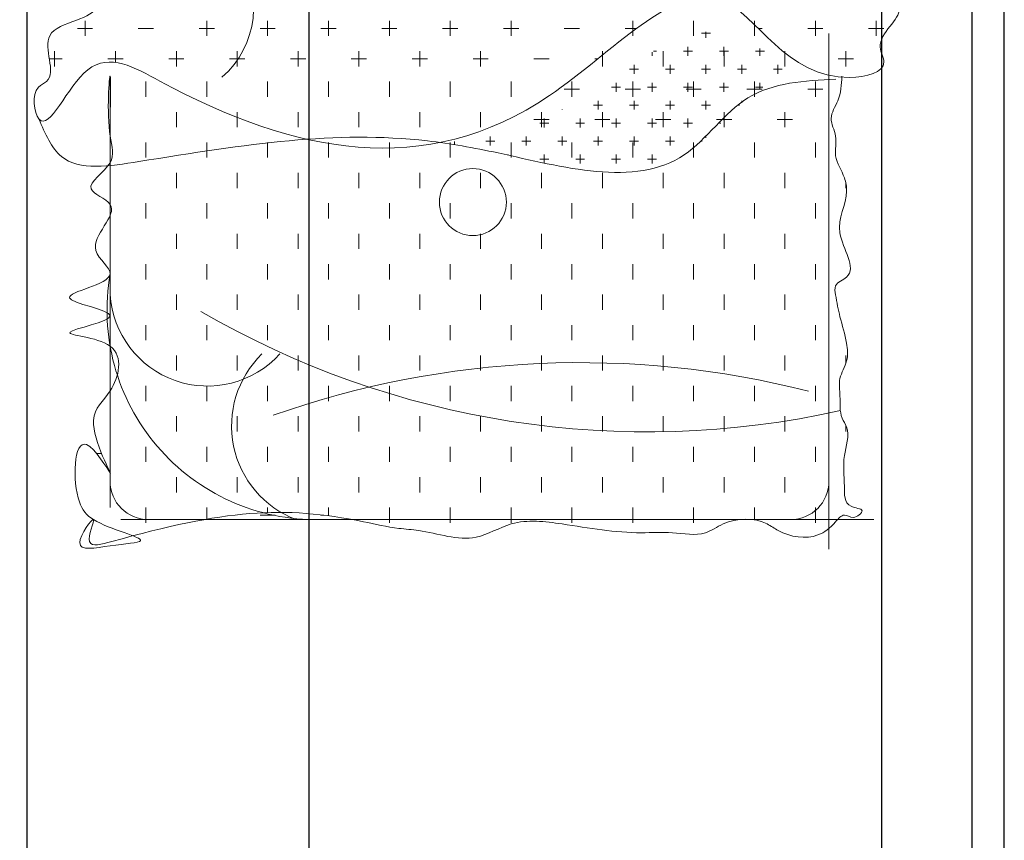
# Model space of a CAD drawing. Units: inches. Extents: x -438 to 102, y -60 to 1091.
# Tile 16 of 20: x -68 to 13, y 699 to 766. Entities that reach past the tile are written whole.
import ezdxf

# ---------------------------------------------------------------- set-up
doc = ezdxf.new("R2010")
doc.units = ezdxf.units.IN
doc.header["$MEASUREMENT"] = 0
doc.layers.add('A-ANNO-DIMS', color=217, linetype='Continuous', lineweight=18, true_color=0x93278f)
doc.layers.add('Furniture', color=7, linetype='Continuous', lineweight=15)
doc.styles.get("Standard").update_dxf_attribs({"font": 'arial.ttf'})
doc.dimstyles.get("Standard").update_dxf_attribs({"dimtxt": 8, "dimasz": 0.18, "dimexe": 0.18, "dimexo": 0.0625, "dimgap": 0.09, "dimtad": 0, "dimtih": 1, "dimtoh": 1, "dimdec": 4, "dimzin": 0, "dimdsep": 46, "dimlunit": 3, "dimtxsty": 'Standard', "dimcen": 0.09, "dimadec": 0, "dimazin": 0, "dimtfac": 1, "dimtdec": 4, "dimtofl": 0, "dimtmove": 0, "dimatfit": 3, "dimfxl": 1, "dimtolj": 1, "dimtzin": 0, "dimarcsym": 0})

# ---------------------------------------------------------------- blocks, each defined once
blk = doc.blocks.new('BED-DOUBLE-WITH-NIGHTSTANDS')
for p, q in [((-31.218, -41.19), (-31.218, -39.94)), ((-21.218, -41.19), (-21.218, -39.94)), ((-16.218, -41.19), (-16.218, -39.94)), ((-11.218, -41.19), (-11.218, -39.94)), ((-6.218, -41.19), (-6.218, -39.94)), ((-1.218, -41.19), (-1.218, -39.94)), ((3.782, -41.19), (3.782, -39.94)), ((13.782, -41.19), (13.782, -39.94)), ((18.782, -41.19), (18.782, -39.94)), ((23.782, -41.19), (23.782, -39.94)), ((28.782, -41.19), (28.782, -39.94)), ((33.782, -41.19), (33.782, -39.94)), ((-30.593, -40.565), (-31.843, -40.565)), ((-25.593, -40.565), (-26.843, -40.565)), ((-20.593, -40.565), (-21.843, -40.565)), ((-15.593, -40.565), (-16.843, -40.565)), ((-10.593, -40.565), (-11.843, -40.565)), ((-5.593, -40.565), (-6.843, -40.565)), ((-0.593, -40.565), (-1.843, -40.565)), ((4.407, -40.565), (3.157, -40.565)), ((9.407, -40.565), (8.157, -40.565)), ((14.104, -40.565), (13.157, -40.565)), ((20.164, -40.972), (19.426, -40.972)), ((19.795, -41.341), (19.795, -40.863)), ((24.407, -40.565), (24.086, -40.565)), ((29.407, -40.565), (28.157, -40.565)), ((29.898, -40.998), (29.898, -83.358)), ((34.407, -40.565), (33.157, -40.565)), ((-33.718, -43.69), (-33.718, -42.44)), ((-28.718, -43.367), (-28.718, -42.44)), ((-23.718, -43.69), (-23.718, -42.44)), ((-18.718, -43.69), (-18.718, -42.44)), ((-13.718, -43.69), (-13.718, -42.44)), ((-8.718, -43.69), (-8.718, -42.44)), ((-3.718, -43.69), (-3.718, -42.44)), ((1.282, -43.69), (1.282, -42.44)), ((11.282, -43.69), (11.282, -42.44)), ((15.366, -42.817), (15.366, -42.522)), ((15.735, -42.448), (15.495, -42.448)), ((16.282, -43.69), (16.282, -42.44)), ((18.688, -42.448), (17.949, -42.448)), ((18.318, -42.817), (18.318, -42.079)), ((21.64, -42.448), (20.902, -42.448)), ((21.271, -42.817), (21.271, -42.079)), ((21.282, -43.69), (21.282, -42.44)), ((24.593, -42.448), (23.855, -42.448)), ((24.224, -42.817), (24.224, -42.225)), ((26.282, -43.69), (26.282, -42.44)), ((31.282, -43.69), (31.282, -42.44)), ((-33.093, -43.065), (-34.154, -43.065)), ((-28.093, -43.065), (-29.343, -43.065)), ((-23.093, -43.065), (-24.343, -43.065)), ((-18.093, -43.065), (-19.343, -43.065)), ((-13.093, -43.065), (-14.343, -43.065)), ((-8.093, -43.065), (-9.343, -43.065)), ((-3.093, -43.065), (-4.343, -43.065)), ((1.907, -43.065), (0.657, -43.065)), ((6.907, -43.065), (5.657, -43.065)), ((10.916, -43.065), (10.657, -43.065)), ((13.889, -44.294), (13.889, -43.555)), ((16.842, -44.294), (16.842, -43.555)), ((19.795, -44.294), (19.795, -43.555)), ((22.748, -44.294), (22.748, -43.555)), ((25.7, -44.294), (25.7, -43.555)), ((31.907, -43.065), (30.657, -43.065)), ((14.258, -43.924), (13.52, -43.924)), ((17.211, -43.924), (16.473, -43.924)), ((20.164, -43.924), (19.426, -43.924)), ((23.117, -43.924), (22.378, -43.924)), ((26.069, -43.924), (25.331, -43.924)), ((-29.157, -79.94), (-29.157, -44.493)), ((-26.218, -46.19), (-26.218, -44.94)), ((-21.218, -46.19), (-21.218, -44.94)), ((-16.218, -46.19), (-16.218, -44.94)), ((-11.218, -46.19), (-11.218, -44.94)), ((-6.218, -46.19), (-6.218, -44.94)), ((-1.218, -46.19), (-1.218, -44.94)), ((3.782, -46.19), (3.782, -44.94)), ((8.782, -46.19), (8.782, -44.94)), ((12.413, -45.77), (12.413, -45.032)), ((13.782, -46.19), (13.782, -44.94)), ((15.366, -45.77), (15.366, -45.032)), ((18.318, -45.77), (18.318, -45.032)), ((18.782, -46.19), (18.782, -44.94)), ((21.271, -45.77), (21.271, -45.032)), ((23.782, -46.19), (23.782, -44.94)), ((24.224, -45.56), (24.224, -45.032)), ((28.782, -46.19), (28.782, -44.94)), ((9.407, -45.565), (8.157, -45.565)), ((12.782, -45.401), (12.044, -45.401)), ((14.407, -45.565), (13.157, -45.565)), ((15.735, -45.401), (14.997, -45.401)), ((18.688, -45.401), (17.949, -45.401)), ((19.407, -45.565), (18.157, -45.565)), ((21.64, -45.401), (20.902, -45.401)), ((24.407, -45.565), (23.157, -45.565)), ((24.466, -45.401), (23.855, -45.401)), ((29.407, -45.565), (28.157, -45.565)), ((11.306, -46.877), (10.567, -46.877)), ((10.937, -47.246), (10.937, -46.508)), ((14.258, -46.877), (13.52, -46.877)), ((13.889, -47.246), (13.889, -46.508)), ((17.211, -46.877), (16.473, -46.877)), ((16.842, -47.246), (16.842, -46.508)), ((20.164, -46.877), (19.426, -46.877)), ((19.795, -47.246), (19.795, -46.508)), ((22.546, -46.877), (22.378, -46.877)), ((22.748, -46.697), (22.748, -46.508)), ((-23.718, -48.69), (-23.718, -47.44)), ((-18.718, -48.69), (-18.718, -47.44)), ((-13.718, -48.69), (-13.718, -47.44)), ((-8.718, -48.69), (-8.718, -47.44)), ((-3.718, -48.69), (-3.718, -47.44)), ((1.282, -48.69), (1.282, -47.44)), ((6.282, -48.69), (6.282, -47.44)), ((7.984, -47.246), (7.984, -47.199)), ((11.282, -48.69), (11.282, -47.44)), ((16.282, -48.69), (16.282, -47.44)), ((21.282, -48.69), (21.282, -47.44)), ((26.282, -48.69), (26.282, -47.44)), ((-34.327, -48.065), (-34.343, -48.065)), ((6.907, -48.065), (5.657, -48.065)), ((6.877, -48.354), (6.138, -48.354)), ((6.507, -48.723), (6.507, -47.984)), ((9.829, -48.354), (9.091, -48.354)), ((9.46, -48.723), (9.46, -47.984)), ((11.907, -48.065), (10.657, -48.065)), ((12.782, -48.354), (12.044, -48.354)), ((12.413, -48.723), (12.413, -47.984)), ((15.735, -48.354), (14.997, -48.354)), ((15.366, -48.723), (15.366, -47.984)), ((16.907, -48.065), (15.657, -48.065)), ((18.688, -48.354), (17.949, -48.354)), ((18.318, -48.723), (18.318, -47.984)), ((21.907, -48.065), (20.657, -48.065)), ((21.024, -48.354), (20.902, -48.354)), ((21.271, -48.106), (21.271, -47.984)), ((26.907, -48.065), (25.657, -48.065)), ((-26.218, -51.19), (-26.218, -49.94)), ((-21.218, -51.19), (-21.218, -49.94)), ((-16.218, -51.19), (-16.218, -49.94)), ((-11.218, -51.19), (-11.218, -49.94)), ((-6.218, -51.19), (-6.218, -49.94)), ((-1.218, -51.19), (-1.218, -49.94)), ((-0.874, -50.112), (-0.874, -49.874)), ((2.447, -49.83), (1.709, -49.83)), ((2.078, -50.199), (2.078, -49.461)), ((3.782, -51.19), (3.782, -49.94)), ((5.4, -49.83), (4.662, -49.83)), ((5.031, -50.199), (5.031, -49.461)), ((8.353, -49.83), (7.615, -49.83)), ((7.984, -50.199), (7.984, -49.461)), ((8.782, -51.19), (8.782, -49.94)), ((11.306, -49.83), (10.567, -49.83)), ((10.937, -50.199), (10.937, -49.461)), ((14.258, -49.83), (13.52, -49.83)), ((13.782, -51.19), (13.782, -49.94)), ((13.889, -50.199), (13.889, -49.461)), ((17.211, -49.83), (16.473, -49.83)), ((16.842, -50.199), (16.842, -49.461)), ((18.782, -51.19), (18.782, -49.94)), ((19.485, -49.83), (19.426, -49.83)), ((19.795, -49.55), (19.795, -49.461)), ((23.782, -51.19), (23.782, -49.94)), ((28.782, -51.19), (28.782, -49.94)), ((3.555, -50.987), (3.555, -50.937)), ((6.507, -51.614), (6.507, -50.937)), ((9.46, -51.675), (9.46, -50.937)), ((12.413, -51.675), (12.413, -50.937)), ((15.366, -51.675), (15.366, -50.937)), ((6.877, -51.306), (6.138, -51.306)), ((9.829, -51.306), (9.091, -51.306)), ((12.782, -51.306), (12.044, -51.306)), ((15.735, -51.306), (14.997, -51.306)), ((-23.718, -53.69), (-23.718, -52.44)), ((-18.718, -53.69), (-18.718, -52.44)), ((-13.718, -53.69), (-13.718, -52.44)), ((-8.718, -53.69), (-8.718, -52.44)), ((-3.718, -53.69), (-3.718, -52.44)), ((1.282, -53.69), (1.282, -52.44)), ((6.282, -53.69), (6.282, -52.44)), ((11.282, -53.69), (11.282, -52.44)), ((16.282, -53.69), (16.282, -52.44)), ((21.282, -53.69), (21.282, -52.44)), ((26.282, -53.69), (26.282, -52.44)), ((31.282, -53.69), (31.282, -53.251)), ((-26.218, -56.19), (-26.218, -54.94)), ((-21.218, -56.19), (-21.218, -54.94)), ((-16.218, -56.19), (-16.218, -54.94)), ((-11.218, -56.19), (-11.218, -54.94)), ((-6.218, -56.19), (-6.218, -54.94)), ((-1.218, -56.19), (-1.218, -54.94)), ((3.782, -56.19), (3.782, -54.94)), ((8.782, -56.19), (8.782, -54.94)), ((13.782, -56.19), (13.782, -54.94)), ((18.782, -56.19), (18.782, -54.94)), ((23.782, -56.19), (23.782, -54.94)), ((28.782, -56.19), (28.782, -54.94)), ((-23.718, -58.69), (-23.718, -57.44)), ((-18.718, -58.69), (-18.718, -57.44)), ((-13.718, -58.69), (-13.718, -57.44)), ((-8.718, -58.69), (-8.718, -57.44)), ((-3.718, -58.69), (-3.718, -57.44)), ((1.282, -58.69), (1.282, -57.44)), ((6.282, -58.69), (6.282, -57.44)), ((11.282, -58.69), (11.282, -57.44)), ((16.282, -58.69), (16.282, -57.44)), ((21.282, -58.69), (21.282, -57.44)), ((26.282, -58.69), (26.282, -57.44)), ((-26.218, -61.19), (-26.218, -59.94)), ((-21.218, -61.19), (-21.218, -59.94)), ((-16.218, -61.19), (-16.218, -59.94)), ((-11.218, -61.19), (-11.218, -59.94)), ((-6.218, -61.19), (-6.218, -59.94)), ((-1.218, -61.19), (-1.218, -59.94)), ((3.782, -61.19), (3.782, -59.94)), ((8.782, -61.19), (8.782, -59.94)), ((13.782, -61.19), (13.782, -59.94)), ((18.782, -61.19), (18.782, -59.94)), ((23.782, -61.19), (23.782, -59.94)), ((28.782, -61.19), (28.782, -59.94)), ((-23.718, -63.69), (-23.718, -62.44)), ((-18.718, -63.69), (-18.718, -62.44)), ((-13.718, -63.69), (-13.718, -62.44)), ((-8.718, -63.69), (-8.718, -62.44)), ((-3.718, -63.69), (-3.718, -62.44)), ((1.282, -63.69), (1.282, -62.44)), ((6.282, -63.69), (6.282, -62.44)), ((11.282, -63.69), (11.282, -62.44)), ((16.282, -63.69), (16.282, -62.44)), ((21.282, -63.69), (21.282, -62.44)), ((26.282, -63.69), (26.282, -62.44)), ((-26.218, -66.19), (-26.218, -64.94)), ((-21.218, -66.19), (-21.218, -64.94)), ((-16.218, -66.19), (-16.218, -64.94)), ((-11.218, -66.19), (-11.218, -64.94)), ((-6.218, -66.19), (-6.218, -64.94)), ((-1.218, -66.19), (-1.218, -64.94)), ((3.782, -66.19), (3.782, -64.94)), ((8.782, -66.19), (8.782, -64.94)), ((13.782, -66.19), (13.782, -64.94)), ((18.782, -66.19), (18.782, -64.94)), ((23.782, -66.19), (23.782, -64.94)), ((28.782, -66.19), (28.782, -64.94)), ((-23.718, -68.69), (-23.718, -67.44)), ((-18.718, -68.69), (-18.718, -67.44)), ((-13.718, -68.69), (-13.718, -67.44)), ((-8.718, -68.69), (-8.718, -67.44)), ((-3.718, -68.69), (-3.718, -67.44)), ((1.282, -68.69), (1.282, -67.44)), ((6.282, -68.69), (6.282, -67.44)), ((11.282, -68.69), (11.282, -67.44)), ((16.282, -68.69), (16.282, -67.44)), ((21.282, -68.69), (21.282, -67.44)), ((26.282, -68.69), (26.282, -67.44)), ((31.282, -68.103), (31.282, -67.44)), ((-26.218, -71.19), (-26.218, -69.94)), ((-21.218, -71.19), (-21.218, -69.94)), ((-16.218, -71.19), (-16.218, -69.94)), ((-11.218, -71.19), (-11.218, -69.94)), ((-6.218, -71.19), (-6.218, -69.94)), ((-1.218, -71.19), (-1.218, -69.94)), ((3.782, -71.19), (3.782, -69.94)), ((8.782, -71.19), (8.782, -69.94)), ((13.782, -71.19), (13.782, -69.94)), ((18.782, -71.19), (18.782, -69.94)), ((23.782, -71.19), (23.782, -69.94)), ((28.782, -71.19), (28.782, -69.94)), ((-23.718, -73.69), (-23.718, -72.44)), ((-18.718, -73.69), (-18.718, -72.44)), ((-13.718, -73.69), (-13.718, -72.44)), ((-8.718, -73.69), (-8.718, -72.44)), ((-3.718, -73.69), (-3.718, -72.44)), ((1.282, -73.69), (1.282, -72.44)), ((6.282, -73.69), (6.282, -72.44)), ((11.282, -73.69), (11.282, -72.44)), ((16.282, -73.69), (16.282, -72.44)), ((21.282, -73.69), (21.282, -72.44)), ((26.282, -73.69), (26.282, -72.44)), ((31.282, -73.69), (31.282, -73.162)), ((-26.218, -76.19), (-26.218, -74.94)), ((-21.218, -76.19), (-21.218, -74.94)), ((-16.218, -76.19), (-16.218, -74.94)), ((-11.218, -76.19), (-11.218, -74.94)), ((-6.218, -76.19), (-6.218, -74.94)), ((-1.218, -76.19), (-1.218, -74.94)), ((3.782, -76.19), (3.782, -74.94)), ((8.782, -76.19), (8.782, -74.94)), ((13.782, -76.19), (13.782, -74.94)), ((18.782, -76.19), (18.782, -74.94)), ((23.782, -76.19), (23.782, -74.94)), ((28.782, -76.19), (28.782, -74.94)), ((-29.87, -75.491), (-30.279, -75.491)), ((-23.718, -78.69), (-23.718, -77.44)), ((-18.718, -78.69), (-18.718, -77.44)), ((-13.718, -78.69), (-13.718, -77.44)), ((-8.718, -78.69), (-8.718, -77.44)), ((-3.718, -78.69), (-3.718, -77.44)), ((1.282, -78.69), (1.282, -77.44)), ((6.282, -78.69), (6.282, -77.44)), ((11.282, -78.69), (11.282, -77.44)), ((16.282, -78.69), (16.282, -77.44)), ((21.282, -78.69), (21.282, -77.44)), ((26.282, -78.69), (26.282, -77.44)), ((-26.218, -81.19), (-26.218, -79.94)), ((-21.218, -80.893), (-21.218, -79.94)), ((-16.218, -80.354), (-16.218, -79.94)), ((-11.218, -80.612), (-11.218, -79.94)), ((-6.218, -81.19), (-6.218, -79.94)), ((-1.218, -81.19), (-1.218, -79.94)), ((3.782, -81.19), (3.782, -79.94)), ((8.782, -81.19), (8.782, -79.94)), ((13.782, -81.19), (13.782, -79.94)), ((18.782, -81.19), (18.782, -79.94)), ((23.782, -80.944), (23.782, -79.94)), ((28.782, -81.19), (28.782, -79.94)), ((-15.593, -80.565), (-16.843, -80.565)), ((-11.59, -80.565), (-11.843, -80.565)), ((33.596, -80.928), (-28.288, -80.928))]:
    blk.add_line(p, q)
blk.add_circle((0.643, -54.842), 2.753)
for centre, radius, start, end in [((-24.929, -38.89), 7.557, 311.04012, 36.13845), ((-12.201, -63.717), 17.214, 170.06779, 270.93205), ((-21.159, -61.944), 8.013, 183.53609, 317.84857), ((14.986, -0.753), 72.965, 239.8126, 282.54723), ((-10.938, -73.228), 8.244, 134.23532, 249.05847), ((9.498, -143.884), 75.853, 75.71433, 109.44594), ((-26.01, -77.778), 3.15, 180, 270), ((26.749, -77.778), 3.15, 270, 0)]:
    blk.add_arc(centre, radius, start, end)
for points, knots in [([(31.925, -25.289), (32.572, -26.623), (33.591, -28.721), (30.294, -29.708), (31.006, -32.636), (33.349, -32.829), (32.919, -35.123), (30.078, -36.111), (33.789, -37.483), (36.776, -39.184), (33.388, -41.323), (35.068, -44.058), (26.871, -46.019), (20.992, -32.347), (2.098, -54.118), (-16.077, -50.434), (-31.165, -41.37), (-34.819, -50.791), (-35.745, -45.559), (-33.272, -44.571), (-36.072, -39.916), (-29.615, -39.911), (-31.051, -37.176), (-31.793, -35.409), (-31.667, -30.426), (-16.859, -30.756), (-35.732, -24.414), (-25.676, -23.879), (-16.82, -24.973), (2.336, -26.688), (17.46, -24.9), (30.087, -22.482), (31.544, -24.706), (31.925, -25.289)], [0, 0, 0, 0, 3.481099, 5.475811, 8.043407, 9.436812, 11.330727, 12.888379, 16.258255, 18.252967, 21.734596, 23.018392, 26.087149, 38.445812, 54.5649, 86.600283, 92.594507, 98.286547, 100.905288, 101.70342, 105.471876, 109.954916, 110.954151, 113.598333, 116.114301, 124.231953, 133.25029, 137.509046, 143.991555, 164.906349, 189.961005, 195.579007, 197.573325, 197.573325, 197.573325, 197.573325]), ([(30.963, -44.508), (30.926, -45.187), (30.862, -46.385), (29.771, -47.932), (30.68, -49.438), (30.181, -51.195), (31.183, -52.546), (31.556, -54.753), (29.857, -57.224), (32.609, -60.735), (30.283, -61.502), (30.515, -62.875), (30.787, -64.379), (31.375, -66.149), (31.511, -67.951), (30.622, -69.27), (30.889, -70.902), (30.721, -72.32), (31.738, -73.744), (30.928, -75.806), (31.246, -77.781), (31.095, -79.972), (33.091, -80.014), (31.893, -81.001), (31.103, -80.322), (30.205, -81.428), (28.73, -82.665), (26.29, -82.307), (24.174, -80.727), (21.697, -80.779), (19.495, -82.403), (17.064, -81.884), (13.167, -82.166), (8.822, -81.359), (4.068, -80.767), (0.461, -83.087), (-2.79, -81.846), (-5.869, -81.655), (-14.296, -79.687), (-20.145, -80.176), (-31.546, -83.45), (-29.775, -79.604), (-32.809, -83.796), (-29.072, -82.964), (-24.845, -82.73), (-30.357, -81.504), (-32.306, -79.089), (-32.112, -72.198), (-27.723, -79.522), (-31.689, -72.602), (-28.723, -70.506), (-27.651, -65.929), (-35.205, -65.768), (-26.021, -64.125), (-35.787, -62.68), (-27.319, -61.348), (-31.947, -58.401), (-27.389, -55.207), (-31.953, -53.756), (-28.502, -51.755), (-29.554, -48.806), (-29.069, -42.18), (-29.131, -46.294), (-29.157, -48.01)], [0, 0, 0, 0, 2.033881, 3.581387, 5.07489, 6.704853, 8.655612, 9.757262, 13.24098, 16.903694, 18.063816, 18.788243, 20.635227, 22.875483, 24.324336, 25.871843, 27.320698, 29.140811, 29.950855, 32.312207, 34.847704, 36.565952, 37.541804, 38.447727, 39.194923, 40.100844, 41.912688, 45.194843, 46.251388, 49.875946, 51.496686, 54.215105, 56.7523, 63.316606, 67.484853, 70.581422, 75.324573, 76.965649, 79.915763, 100.671038, 102.483321, 104.317501, 106.523635, 109.038061, 111.571263, 115.809372, 117.667229, 122.411431, 125.445794, 129.976907, 132.758854, 136.424739, 139.918708, 143.481583, 147.135325, 151.002466, 153.252794, 157.23352, 159.244583, 161.905351, 164.097269, 169.015093, 172.531686, 172.531686, 172.531686, 172.531686]), ([(30.466, -44.728), (27.876, -44.872), (22.825, -45.152), (16.718, -54.501), (5.643, -51.254), (-8.894, -48.66), (-19.851, -50.381), (-33.096, -52.536), (-34.5, -49.206), (-35.005, -48.009)], [0, 0, 0, 0, 7.385187, 14.402621, 29.694422, 35.583277, 59.348121, 65.733553, 69.320983, 69.320983, 69.320983, 69.320983])]:
    blk.add_open_spline(points, degree=3, knots=knots)
blk = doc.blocks.new('*D45')
at = {"layer": 'A-ANNO-DIMS', "color": 0, "lineweight": -2, "transparency": 16777216}
for p, q in [((-99.584, 615.92), (-99.584, 1079.579)), ((-99.404, 1079.399), (-59.273, 1079.399)), ((2.316, 1079.399), (-37.816, 1079.399)), ((2.496, 615.92), (2.496, 1079.579))]:
    blk.add_line(p, q, dxfattribs=at)
at = {"layer": 'A-ANNO-DIMS', "color": 0, "transparency": 16777216}
for points in [[(-99.404, 1079.429), (-99.404, 1079.369), (-99.584, 1079.399)], [(2.316, 1079.429), (2.316, 1079.369), (2.496, 1079.399)]]:
    blk.add_solid(points, dxfattribs=at)
at = {"layer": 'Defpoints', "color": 0, "transparency": 16777216}
for p in [(2.496, 1079.399), (-99.584, 615.857), (2.496, 615.857)]:
    blk.add_point(p, dxfattribs=at)
at = {"layer": 'A-ANNO-DIMS', "color": 0, "transparency": 16777216, "insert": (-48.544, 1079.399), "char_height": 8, "attachment_point": 5}
blk.add_mtext('\\A1;8\'-6"', dxfattribs=at)
blk = doc.blocks.new('*D47')
at = {"layer": 'A-ANNO-DIMS', "color": 0, "lineweight": -2, "transparency": 16777216}
for p, q in [((-67.74, 529.328), (-67.74, 1079.579)), ((-67.56, 1079.399), (-48.98, 1079.399)), ((9.731, 1079.399), (-8.849, 1079.399)), ((9.911, 529.328), (9.911, 1079.579))]:
    blk.add_line(p, q, dxfattribs=at)
at = {"layer": 'A-ANNO-DIMS', "color": 0, "transparency": 16777216}
for points in [[(-67.56, 1079.429), (-67.56, 1079.369), (-67.74, 1079.399)], [(9.731, 1079.429), (9.731, 1079.369), (9.911, 1079.399)]]:
    blk.add_solid(points, dxfattribs=at)
at = {"layer": 'Defpoints', "color": 0, "transparency": 16777216}
for p in [(9.911, 1079.399), (-67.74, 529.266), (9.911, 529.266)]:
    blk.add_point(p, dxfattribs=at)
at = {"layer": 'A-ANNO-DIMS', "color": 0, "transparency": 16777216, "insert": (-28.914, 1079.399), "char_height": 8, "attachment_point": 5}
blk.add_mtext('\\A1;6\'-5 1/2"', dxfattribs=at)
blk = doc.blocks.new('*D49')
at = {"layer": 'A-ANNO-DIMS', "color": 0, "lineweight": -2, "transparency": 16777216}
for p, q in [((-44.572, 339.857), (-44.572, 1079.579)), ((-44.392, 1079.399), (-26.894, 1079.399)), ((12.373, 1079.399), (-5.126, 1079.399)), ((12.553, 312.505), (12.553, 1079.579))]:
    blk.add_line(p, q, dxfattribs=at)
at = {"layer": 'A-ANNO-DIMS', "color": 0, "transparency": 16777216}
for points in [[(-44.392, 1079.429), (-44.392, 1079.369), (-44.572, 1079.399)], [(12.373, 1079.429), (12.373, 1079.369), (12.553, 1079.399)]]:
    blk.add_solid(points, dxfattribs=at)
at = {"layer": 'Defpoints', "color": 0, "transparency": 16777216}
for p in [(12.553, 1079.399), (-44.572, 339.795), (12.553, 312.443)]:
    blk.add_point(p, dxfattribs=at)
at = {"layer": 'A-ANNO-DIMS', "color": 0, "transparency": 16777216, "insert": (-16.01, 1079.399), "char_height": 8, "attachment_point": 5}
blk.add_mtext('\\A1;4\'-9"', dxfattribs=at)

msp = doc.modelspace()

# ---------------------------------------------------------------- block references
at = {"layer": 'Furniture'}
msp.add_blockref('BED-DOUBLE-WITH-NIGHTSTANDS', (-31.753, 805.86269), dxfattribs=at)

# ---------------------------------------------------------------- dimensions: what is measured, and where the dimension line sits
at = {"layer": 'A-ANNO-DIMS'}
for base, p1, p2, picture, middle in [((9.9115, 1079.39939), (-67.73982, 529.2655), (9.9115, 529.2655), '*D47', (-28.91416, 1079.39939)), ((2.49567, 1079.39939), (-99.58389, 615.85716), (2.49567, 615.85716), '*D45', (-48.54411, 1079.39939)), ((12.55306, 1079.39939), (-44.57214, 339.79496), (12.55306, 312.44261), '*D49', (-16.00954, 1079.39939))]:
    dim = msp.add_linear_dim(base=base, p1=p1, p2=p2, dimstyle='Standard', override={"dimdec": 1, "dimlfac": 1, "dimrnd": 0, "dimzin": 1, "dimdsep": 46, "dimlunit": 4, "dimfrac": 2}, dxfattribs=at)
    dim.commit()
    dim.dimension.update_dxf_attribs({"geometry": picture, "text_midpoint": middle})

doc.saveas('drawing.dxf')
